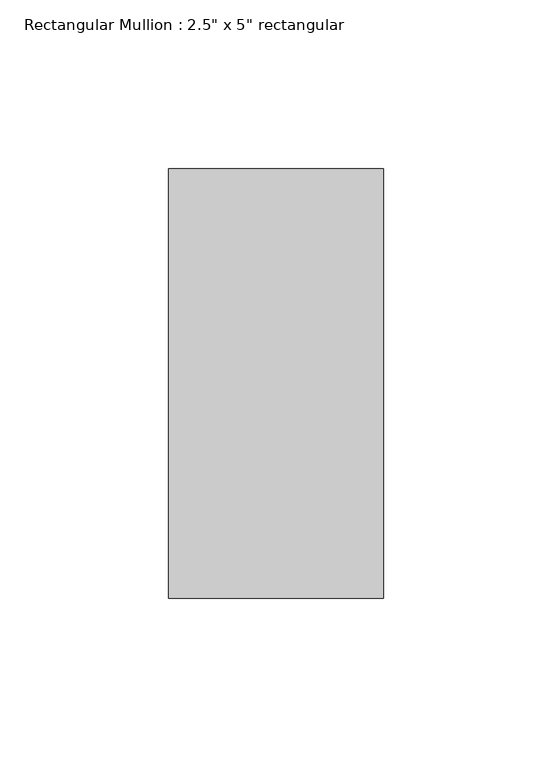
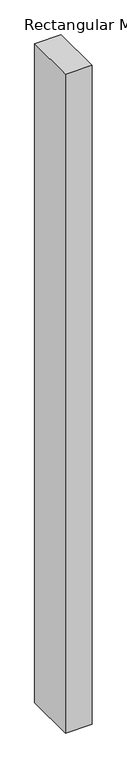
"""IFC4 building model written with IfcOpenShell, lengths in millimetres: member geometry."""

from ifc_helpers import new_model, si_unit, frame, origin, place, context, project, spatial, polyline, outline, extrude, source, transform, mapped, element, save


def member_1e31c4ff(model_context):
    return source(origin(), model_context, "Body", "SweptSolid", [
        extrude(outline(polyline([(31.75, 63.5), (31.75, -63.5), (-31.75, -63.5), (-31.75, 63.5), (31.75, 63.5)])), frame((0.0, 0.0, -1663.8745067), z_axis=(0.0, 0.0, 1.0), x_axis=(1.0, 0.0, 0.0)), (0.0, 0.0, 1.0), 1663.8745067),
    ])


if __name__ == "__main__":
    model = new_model("IFC4")
    model_context = context("Model", 3, world=origin())
    ifc_project = project(units=[si_unit("LENGTHUNIT", "METRE", prefix="MILLI")], contexts=[model_context])
    site = spatial("IfcSite", under=ifc_project)
    building = spatial("IfcBuilding", under=site)
    placement = place(None, origin())
    member_shape = member_1e31c4ff(model_context)
    element("IfcMember", 1, ObjectType="Rectangular Mullion : 2.5\" x 5\" rectangular", at=placement, inside=building, context=model_context, shape_type="MappedRepresentation", body=[
        mapped(member_shape, transform((0.0, 0.0, 0.0), x_axis=(1.0, 0.0, 0.0), y_axis=(0.0, 1.0, 0.0), z_axis=(0.0, 0.0, 1.0))),
    ])
    save(model, "model.ifc")

# Revit data of these elements
# Type "Rectangular Mullion : 2.5\" x 5\" rectangular"
#   built-in parameter 1007304 = 0.416667 (stored number, unit not read)
#   built-in parameter 1007301 = 0.104167 (stored number, unit not read)
#   built-in parameter 1007300 = 0.104167 (stored number, unit not read)
# Element 1 (IfcMember, "Rectangular Mullion : 2.5\" x 5\" rectangular")
#   Materials on its faces: "Aluminum"
# Materials
#   "Aluminum": class "Metal", colour RGB 247 247 247, transparency 0, Description = "Aluminum 6061", Cost = 0
